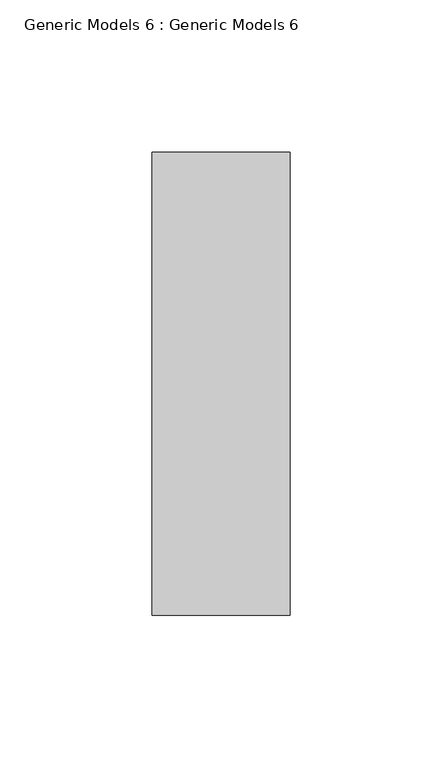
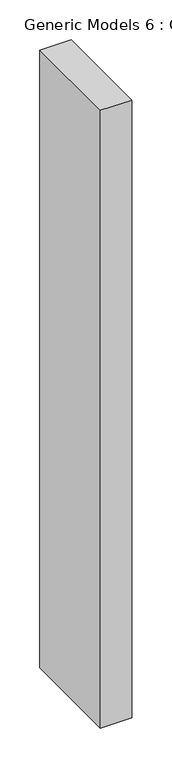
"""IFC4 building model written with IfcOpenShell, lengths in millimetres: proxy geometry, Generic Models 6 : Generic Models 6."""

from ifc_helpers import new_model, si_unit, frame, origin, place, context, project, spatial, polyline, outline, extrude, source, transform, mapped, element, save


def generic_models_6_generic_models_6_594ef515(model_context):
    return source(origin(), model_context, "Body", "SweptSolid", [
        extrude(outline(polyline([(-13059.291855, -13854.1538163), (-13013.8422243, -13854.1538163), (-13013.8422243, -14006.5538163), (-13059.291855, -14006.5538163), (-13059.291855, -13854.1538163)])), frame((0.0, 0.0, 9448.8), z_axis=(0.0, 0.0, 1.0), x_axis=(1.0, 0.0, 0.0)), (0.0, 0.0, 1.0), 946.967225),
    ])


if __name__ == "__main__":
    model = new_model("IFC4")
    model_context = context("Model", 3, world=origin())
    ifc_project = project(units=[si_unit("LENGTHUNIT", "METRE", prefix="MILLI")], contexts=[model_context])
    site = spatial("IfcSite", under=ifc_project)
    building = spatial("IfcBuilding", under=site)
    placement = place(None, origin())
    generic_models_6_generic_models_6_shape = generic_models_6_generic_models_6_594ef515(model_context)
    element("IfcBuildingElementProxy", 1, Name="Generic Models 6 : Generic Models 6", ObjectType="Generic Models 6 : Generic Models 6", at=placement, inside=building, context=model_context, shape_type="MappedRepresentation", body=[
        mapped(generic_models_6_generic_models_6_shape, transform((0.0, 0.0, 0.0), x_axis=(1.0, 0.0, 0.0), y_axis=(0.0, 1.0, 0.0), z_axis=(0.0, 0.0, 1.0))),
    ])
    save(model, "model.ifc")
